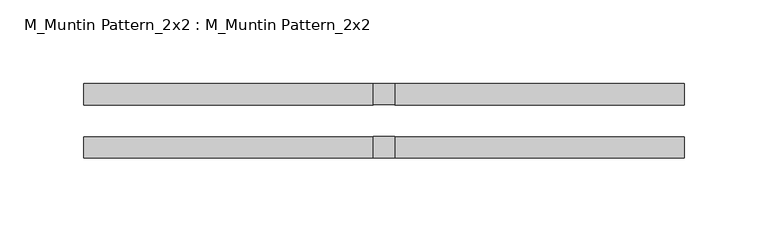
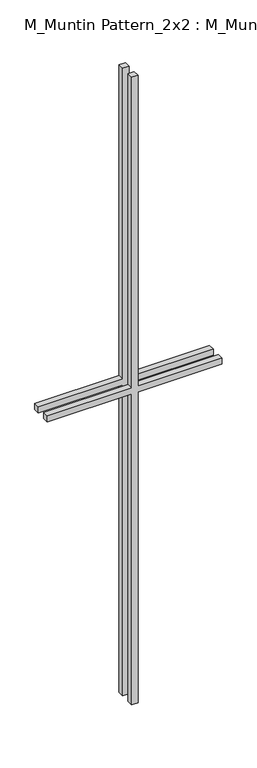
"""IFC4 building model written with IfcOpenShell, lengths in millimetres: proxy geometry, M_Muntin Pattern_2x2 : M_Muntin Pattern_2x2."""

from ifc_helpers import new_model, si_unit, frame, origin, place, context, project, spatial, polyline, outline, extrude, source, transform, mapped, element, save


def m_muntin_pattern_2x2_m_muntin_pattern_2x2_777b163a(model_context):
    return source(origin(), model_context, "Body", "SweptSolid", [
        extrude(outline(polyline([(686.5, -6.35), (686.5, -179.35), (673.8, -179.35), (673.8, -6.35), (0.0, -6.35), (0.0, 6.35), (673.8, 6.35), (673.8, 179.35), (686.5, 179.35), (686.5, 6.35), (1360.3, 6.35), (1360.3, -6.35), (686.5, -6.35)])), frame((0.0, -22.225, 0.0), z_axis=(0.0, 1.0, 0.0), x_axis=(0.0, 0.0, 1.0)), (0.0, 0.0, 1.0), 12.7),
        extrude(outline(polyline([(686.5, -6.35), (686.5, -179.35), (673.8, -179.35), (673.8, -6.35), (0.0, -6.35), (0.0, 6.35), (673.8, 6.35), (673.8, 179.35), (686.5, 179.35), (686.5, 6.35), (1360.3, 6.35), (1360.3, -6.35), (686.5, -6.35)])), frame((0.0, 9.525, 0.0), z_axis=(0.0, 1.0, 0.0), x_axis=(0.0, 0.0, 1.0)), (0.0, 0.0, 1.0), 12.7),
    ])


if __name__ == "__main__":
    model = new_model("IFC4")
    model_context = context("Model", 3, world=origin())
    ifc_project = project(units=[si_unit("LENGTHUNIT", "METRE", prefix="MILLI")], contexts=[model_context])
    site = spatial("IfcSite", under=ifc_project)
    building = spatial("IfcBuilding", under=site)
    placement = place(None, origin())
    m_muntin_pattern_2x2_m_muntin_pattern_2x2_shape = m_muntin_pattern_2x2_m_muntin_pattern_2x2_777b163a(model_context)
    element("IfcBuildingElementProxy", 1, Name="M_Muntin Pattern_2x2 : M_Muntin Pattern_2x2", ObjectType="M_Muntin Pattern_2x2 : M_Muntin Pattern_2x2", at=placement, inside=building, context=model_context, shape_type="MappedRepresentation", body=[
        mapped(m_muntin_pattern_2x2_m_muntin_pattern_2x2_shape, transform((0.0, 0.0, 0.0), x_axis=(1.0, 0.0, 0.0), y_axis=(0.0, 1.0, 0.0), z_axis=(0.0, 0.0, 1.0))),
    ])
    save(model, "model.ifc")

# Revit data of these elements
# Type "M_Muntin Pattern_2x2 : M_Muntin Pattern_2x2"
#   Width [instance default] = 3' - 11.24409"
#   Thickness = 0' - 0 1/2"
#   Height [instance default] = 3' - 11.24409"
#   Distance = 0' - 0 3/4"
#   Interior Material [instance default] = none
#   Exterior Material [instance default] = none
#   Default Elevation = 0
# Element 1 (IfcBuildingElementProxy, "M_Muntin Pattern_2x2 : M_Muntin Pattern_2x2")
#   Width = 1' - 2.12205"
#   Height = 4' - 5.55512"
#   Interior Material = Wood - Stained
#   Exterior Material = Clad - White
#   Materials on its faces: "Clad - White", "Wood - Stained"
# Materials
#   "Clad - White": class "Wood", colour RGB 242 242 238, transparency 0, Cost = 0
#   "Wood - Stained": class "Wood", colour RGB 224 178 126, transparency 0, Cost = 0
